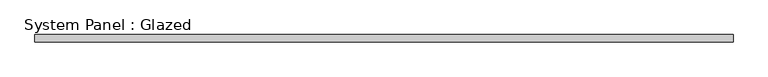
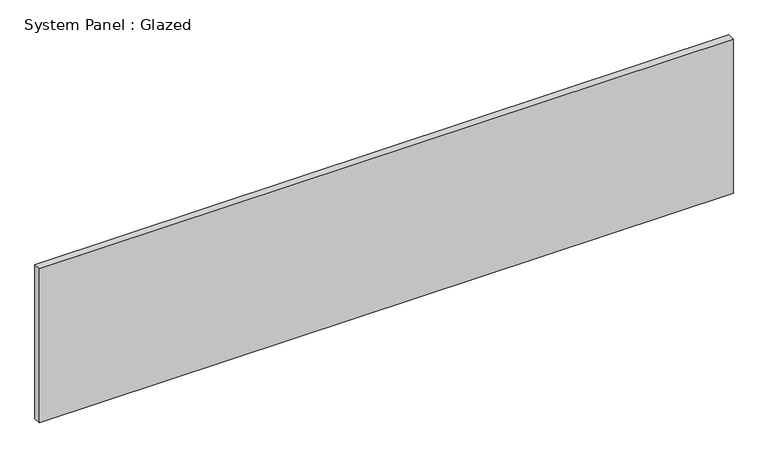
"""IFC4 building model written with IfcOpenShell, lengths in millimetres: plate geometry, System Panel : Glazed."""

from ifc_helpers import new_model, si_unit, origin, origin_with_axes, place, context, project, spatial, polyline, outline, extrude, source, transform, mapped, element, save


def system_panel_glazed_ba5e2c5f(model_context):
    return source(origin(), model_context, "Body", "SweptSolid", [
        extrude(outline(polyline([(1171.575, 19.05), (-1171.575, 19.05), (-1171.575, 44.45), (1171.575, 44.45), (1171.575, 19.05)])), origin_with_axes(), (0.0, 0.0, 1.0), 549.2937999),
    ])


if __name__ == "__main__":
    model = new_model("IFC4")
    model_context = context("Model", 3, world=origin())
    ifc_project = project(units=[si_unit("LENGTHUNIT", "METRE", prefix="MILLI")], contexts=[model_context])
    site = spatial("IfcSite", under=ifc_project)
    building = spatial("IfcBuilding", under=site)
    placement = place(None, origin())
    system_panel_glazed_shape = system_panel_glazed_ba5e2c5f(model_context)
    element("IfcPlate", 1, ObjectType="System Panel : Glazed", at=placement, inside=building, context=model_context, shape_type="MappedRepresentation", body=[
        mapped(system_panel_glazed_shape, transform((0.0, 0.0, 0.0), x_axis=(1.0, 0.0, 0.0), y_axis=(0.0, 1.0, 0.0), z_axis=(0.0, 0.0, 1.0))),
    ])
    save(model, "model.ifc")

# Revit data of these elements
# Type "System Panel : Glazed"
#   Construction Type Id = "GSP4R"
#   Analytic Construction = "1/8 in Pilkington single glazing"
#   Visual Light Transmittance = 0.9
#   Solar Heat Gain Coefficient = 0.86
#   Heat Transfer Coefficient (U) = 1.18115 BTU/(h·ft²·°F)
#   Define Thermal Properties by = 1
# Element 1 (IfcPlate, "System Panel : Glazed")
#   Materials on its faces: "Glass"
# Materials
#   "Glass": class "Glass", colour RGB 0 128 192, transparency 0.75, Description = "Soda Lime Glass", Cost = 0
